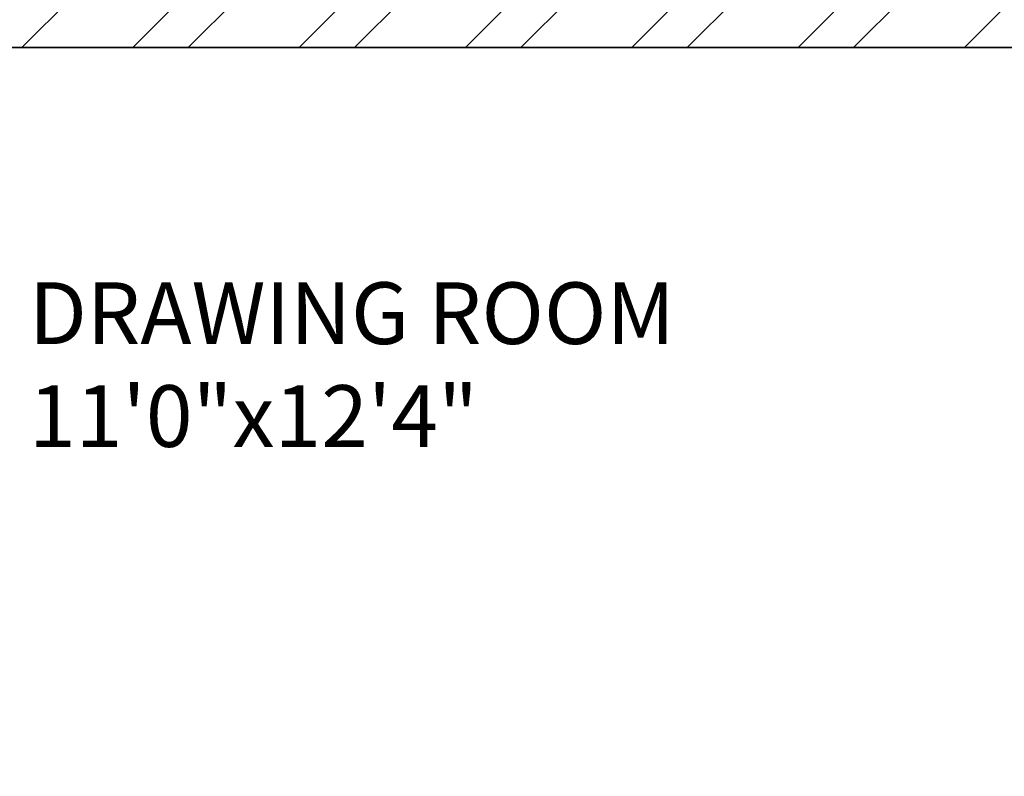
# Model space of a CAD drawing. Units: inches. Extents: x 2168 to 3056, y 1130 to 2629.
# Tile 15 of 42: x 2700 to 2780, y 2017 to 2079. Entities that reach past the tile are written whole.
import ezdxf

# ---------------------------------------------------------------- set-up
doc = ezdxf.new("R2010")
doc.units = ezdxf.units.IN
doc.layers.add('A-AREA-IDEN', color=7, linetype='Continuous', lineweight=18)
doc.layers.add('A-WALL', color=7, linetype='Continuous', lineweight=35)
doc.layers.add('A-WALL-PATT', color=143, linetype='Continuous', lineweight=13, true_color=0x7aafdf)
doc.styles.get("Standard").update_dxf_attribs({"font": 'arial.ttf'})

msp = doc.modelspace()

# ---------------------------------------------------------------- hatches: boundary and pattern name
at = {"layer": 'A-WALL-PATT'}
h = msp.add_hatch(dxfattribs=at)
h.set_pattern_fill('ANSI32', color=256)
h.paths.add_polyline_path([(2463.796, 2409.389), (2467.387, 2409.389), (2467.387, 2413.889), (2454.768, 2413.889), (2454.768, 2411.639), (2454.768, 2409.389), (2459.296, 2409.389), (2459.296, 2265.389), (2455.644, 2265.389), (2455.644, 2260.889), (2467.349, 2260.889), (2467.349, 2263.139), (2467.349, 2265.389), (2463.796, 2265.389)])
h.paths.add_polyline_path([(2431.596, 2413.889), (2409.647, 2413.889), (2409.647, 2409.389), (2431.596, 2409.389), (2431.596, 2411.639)])
h.paths.add_polyline_path([(2349.647, 2413.889), (2331.796, 2413.889), (2331.796, 2362.671), (2336.296, 2362.671), (2336.296, 2409.389), (2349.647, 2409.389), (2349.647, 2411.639)])
h.paths.add_polyline_path([(2634.149, 2411.639), (2634.149, 2413.889), (2562.293, 2413.889), (2562.293, 2409.389), (2595.796, 2409.389), (2595.796, 2280.309), (2595.826, 2280.309), (2595.826, 2265.389), (2499.91, 2265.389), (2499.91, 2260.889), (2550.796, 2260.889), (2550.796, 2117.308), (2555.296, 2117.308), (2555.296, 2168.08), (2571.93, 2168.08), (2571.93, 2176.889), (2559.796, 2176.889), (2559.796, 2256.389), (2640.796, 2256.389), (2640.796, 2176.889), (2626.428, 2176.889), (2626.428, 2168.08), (2645.296, 2168.08), (2645.296, 2116.637), (2649.796, 2116.637), (2649.796, 2260.889), (2691.251, 2260.889), (2691.251, 2263.139), (2691.251, 2265.389), (2670.655, 2265.389), (2670.655, 2265.365), (2600.296, 2265.365), (2600.296, 2280.258), (2600.296, 2409.389), (2634.149, 2409.389)])
h.paths.add_polyline_path([(2600.296, 2473.889), (2612.84, 2473.889), (2612.84, 2478.389), (2572.636, 2478.389), (2572.636, 2473.889), (2595.796, 2473.889), (2595.796, 2413.889), (2600.296, 2413.889)])
h.paths.add_polyline_path([(2535.796, 2473.889), (2548.636, 2473.889), (2548.636, 2478.389), (2531.396, 2478.389), (2531.396, 2413.889), (2521.6, 2413.889), (2521.6, 2409.389), (2539.239, 2409.389), (2539.239, 2411.639), (2539.239, 2413.889), (2535.796, 2413.889)])
h.paths.add_polyline_path([(2664.796, 2478.389), (2636.84, 2478.389), (2636.84, 2473.889), (2660.296, 2473.889), (2660.296, 2413.889), (2656.165, 2413.889), (2656.165, 2409.389), (2671.684, 2409.389), (2671.684, 2411.639), (2671.684, 2413.889), (2664.796, 2413.889)])
h.paths.add_polyline_path([(2705.942, 2413.889), (2695.684, 2413.889), (2695.684, 2409.389), (2705.942, 2409.389)])
h.paths.add_polyline_path([(2741.35, 2413.889), (2728.733, 2413.889), (2728.733, 2411.639), (2728.733, 2409.389), (2732.296, 2409.389), (2732.296, 2265.389), (2725.733, 2265.389), (2725.733, 2260.889), (2740.917, 2260.889), (2740.917, 2263.139), (2740.917, 2265.389), (2736.796, 2265.389), (2736.796, 2409.389), (2741.35, 2409.389)])
h.paths.add_polyline_path([(2785.655, 2413.889), (2764.546, 2413.889), (2764.486, 2409.389), (2785.655, 2409.389), (2785.655, 2411.639)])
h.paths.add_polyline_path([(2864.296, 2413.889), (2845.655, 2413.889), (2845.655, 2409.389), (2859.796, 2409.389), (2859.796, 2368.425), (2864.296, 2368.425)])
h.paths.add_polyline_path([(2864.296, 2308.425), (2862.046, 2308.425), (2859.796, 2308.425), (2859.796, 2265.389), (2774.483, 2265.389), (2774.483, 2263.139), (2774.483, 2260.889), (2781.796, 2260.889), (2781.796, 2226.654), (2786.296, 2226.654), (2786.296, 2260.889), (2859.796, 2260.889), (2859.796, 2241.352), (2864.296, 2241.352)])
h.paths.add_polyline_path([(2864.296, 2217.352), (2862.046, 2217.352), (2859.796, 2217.352), (2859.796, 2200.889), (2786.296, 2200.889), (2786.296, 2205.931), (2784.046, 2205.931), (2781.796, 2205.931), (2781.796, 2150.974), (2786.296, 2150.974), (2786.296, 2161.889), (2859.796, 2161.889), (2859.796, 2144.419), (2864.296, 2144.419)])
h.paths.add_polyline_path([(2859.796, 2196.389), (2859.796, 2166.389), (2786.296, 2166.389), (2786.296, 2196.389)], flags=16)
h.paths.add_polyline_path([(2864.296, 2108.419), (2862.046, 2108.419), (2859.796, 2108.419), (2859.796, 2080.889), (2786.296, 2080.889), (2786.296, 2111.993), (2781.796, 2111.993), (2781.796, 2080.889), (2649.796, 2080.889), (2649.796, 2086.036), (2647.546, 2086.036), (2645.296, 2086.036), (2645.296, 2071.739), (2649.796, 2071.739), (2649.796, 2076.389), (2781.796, 2076.389), (2781.796, 2041.792), (2786.296, 2041.792), (2786.296, 2076.389), (2859.796, 2076.389), (2859.796, 2058.577), (2864.296, 2058.577)])
h.paths.add_polyline_path([(2864.296, 2022.577), (2859.796, 2022.577), (2859.796, 1992.389), (2786.296, 1992.389), (2786.296, 1999.573), (2781.796, 1999.573), (2781.796, 1848.085), (2784.046, 1848.085), (2786.296, 1848.085), (2786.296, 1851.389), (2859.796, 1851.389), (2859.796, 1838.258), (2864.296, 1838.258)], flags=17)
h.paths.add_polyline_path([(2859.796, 1987.889), (2859.796, 1855.889), (2786.296, 1855.889), (2786.296, 1987.889)], flags=16)
h.paths.add_polyline_path([(2823.046, 1987.889), (2841.421, 1921.889), (2823.046, 1855.889)], flags=0)
h.paths.add_polyline_path([(2864.296, 1814.258), (2859.796, 1814.258), (2859.796, 1791.389), (2786.296, 1791.389), (2786.296, 1825.658), (2784.046, 1825.658), (2781.796, 1825.658), (2781.796, 1791.389), (2720.155, 1791.389), (2720.155, 1791.265), (2649.796, 1791.265), (2649.796, 1806.159), (2649.796, 2038.983), (2647.546, 2038.983), (2645.296, 2038.983), (2645.296, 1783.925), (2649.796, 1783.925), (2649.796, 1786.889), (2781.796, 1786.889), (2781.796, 1746.789), (2786.296, 1746.789), (2786.296, 1786.889), (2859.796, 1786.889), (2859.796, 1770.083), (2864.296, 1770.083)])
h.paths.add_polyline_path([(2864.296, 1734.083), (2862.046, 1734.083), (2859.796, 1734.083), (2859.796, 1705.889), (2786.296, 1705.889), (2786.296, 1714.166), (2781.796, 1714.166), (2781.796, 1660.527), (2786.296, 1660.527), (2786.296, 1666.889), (2859.796, 1666.889), (2859.796, 1648.342), (2864.296, 1648.342)])
h.paths.add_polyline_path([(2786.296, 1701.389), (2859.796, 1701.389), (2859.796, 1671.389), (2786.296, 1671.389)], flags=16)
h.paths.add_polyline_path([(2649.796, 1756.576), (2647.546, 1756.576), (2645.296, 1756.576), (2645.296, 1606.889), (2555.296, 1606.889), (2555.296, 1749.513), (2553.046, 1749.513), (2550.796, 1749.513), (2550.796, 1606.889), (2503.006, 1606.889), (2503.006, 1604.639), (2503.006, 1602.389), (2595.796, 1602.389), (2595.849, 1602.389), (2595.849, 1587.495), (2595.796, 1458.389), (2561.502, 1458.389), (2561.502, 1456.139), (2561.502, 1453.889), (2595.796, 1453.889), (2595.796, 1381.889), (2573.438, 1381.889), (2573.438, 1377.389), (2613.01, 1377.389), (2613.01, 1379.639), (2613.01, 1381.889), (2600.296, 1381.889), (2600.296, 1453.889), (2634.327, 1453.889), (2634.327, 1458.389), (2600.296, 1458.389), (2600.296, 1602.389), (2670.655, 1602.389), (2694.095, 1602.389), (2694.095, 1606.889), (2649.796, 1606.889)])
h.paths.add_polyline_path([(2736.796, 1602.389), (2741.562, 1602.389), (2741.562, 1606.889), (2726.203, 1606.889), (2726.203, 1604.639), (2726.203, 1602.389), (2732.296, 1602.389), (2732.296, 1458.389), (2727.899, 1458.389), (2727.899, 1453.889), (2740.821, 1453.889), (2740.821, 1456.139), (2740.821, 1458.389), (2736.796, 1458.389)])
h.paths.add_polyline_path([(2859.796, 1606.889), (2786.296, 1606.889), (2786.296, 1637.334), (2784.046, 1637.334), (2781.796, 1637.334), (2781.796, 1606.889), (2775.612, 1606.889), (2775.612, 1602.389), (2859.796, 1602.389)])
h.paths.add_polyline_path([(2864.296, 1624.342), (2862.046, 1624.342), (2859.796, 1624.342), (2859.796, 1570.39), (2864.296, 1570.39)])
h.paths.add_polyline_path([(2864.296, 1510.39), (2862.046, 1510.39), (2859.796, 1510.39), (2859.796, 1458.389), (2846.735, 1458.389), (2846.735, 1456.139), (2846.735, 1453.889), (2864.296, 1453.889)])
h.paths.add_polyline_path([(2786.735, 1458.389), (2765.444, 1458.389), (2765.444, 1453.889), (2786.735, 1453.889)])
h.paths.add_polyline_path([(2706.004, 1458.389), (2695.36, 1458.389), (2695.36, 1453.889), (2706.004, 1453.889), (2706.004, 1456.139)])
h.paths.add_polyline_path([(2671.36, 1456.139), (2671.36, 1458.389), (2655.986, 1458.389), (2655.986, 1456.139), (2655.986, 1453.889), (2660.296, 1453.889), (2660.296, 1381.889), (2637.01, 1381.889), (2637.01, 1377.389), (2664.796, 1377.389), (2664.796, 1453.889), (2671.36, 1453.889)], flags=17)
h.paths.add_polyline_path([(2539.829, 1458.389), (2520.237, 1458.389), (2520.237, 1453.889), (2531.296, 1453.889), (2531.296, 1377.389), (2546.449, 1377.389), (2546.449, 1379.639), (2546.449, 1381.889), (2535.796, 1381.889), (2535.796, 1453.889), (2539.829, 1453.889)], flags=17)
h.paths.add_polyline_path([(2496.237, 1458.389), (2489.13, 1458.389), (2489.13, 1453.889), (2496.237, 1453.889), (2496.237, 1456.139)])
h.paths.add_polyline_path([(2467.433, 1456.139), (2467.433, 1458.389), (2463.796, 1458.389), (2463.796, 1602.389), (2468.242, 1602.389), (2468.242, 1605.7), (2468.242, 1606.889), (2454.602, 1606.889), (2454.602, 1602.389), (2459.296, 1602.389), (2459.296, 1458.389), (2454.24, 1458.389), (2454.24, 1453.889), (2467.433, 1453.889)])
h.paths.add_polyline_path([(2431.601, 1456.139), (2431.601, 1458.389), (2411.386, 1458.389), (2411.386, 1453.889), (2431.601, 1453.889)])
h.paths.add_polyline_path([(2351.386, 1458.389), (2336.296, 1458.389), (2336.296, 1490.693), (2334.046, 1490.693), (2331.796, 1490.693), (2331.796, 1453.889), (2351.386, 1453.889), (2351.386, 1456.139)])
h.paths.add_polyline_path([(2336.296, 1629.705), (2331.796, 1629.705), (2331.796, 1552.317), (2336.296, 1552.317), (2336.296, 1602.389), (2406.655, 1602.389), (2423.472, 1602.389), (2423.472, 1606.889), (2418.796, 1606.889), (2418.796, 1643.678), (2416.546, 1643.678), (2414.296, 1643.678), (2414.296, 1606.889), (2336.296, 1606.889)])
h.paths.add_polyline_path([(2418.796, 1714.384), (2414.296, 1714.384), (2414.296, 1705.889), (2336.296, 1705.889), (2336.296, 1731.324), (2334.046, 1731.324), (2331.796, 1731.324), (2331.796, 1653.705), (2334.046, 1653.705), (2336.296, 1653.705), (2336.296, 1666.889), (2414.296, 1666.889), (2414.296, 1663.589), (2418.796, 1663.589)])
h.paths.add_polyline_path([(2336.296, 1701.389), (2414.296, 1701.389), (2414.296, 1671.389), (2336.296, 1671.389)], flags=16)
h.paths.add_polyline_path([(2555.296, 2040.059), (2550.796, 2040.059), (2550.796, 1791.389), (2550.561, 1791.205), (2480.202, 1791.205), (2418.796, 1791.389), (2418.796, 1825.448), (2416.546, 1825.448), (2414.296, 1825.448), (2414.296, 1791.389), (2336.296, 1791.389), (2336.296, 1806.409), (2331.796, 1806.409), (2331.796, 1767.324), (2336.296, 1767.324), (2336.296, 1786.889), (2414.296, 1786.889), (2414.296, 1745.457), (2418.796, 1745.457), (2418.796, 1786.889), (2550.796, 1786.889), (2550.796, 1783.011), (2555.296, 1783.011)])
h.paths.add_polyline_path([(2418.796, 1923.389), (2423.207, 1923.389), (2423.207, 1925.639), (2423.207, 1927.889), (2418.796, 1927.889), (2418.796, 2000.048), (2414.296, 2000.048), (2414.296, 1992.389), (2336.296, 1992.389), (2336.296, 1987.889), (2414.296, 1987.889), (2414.296, 1855.889), (2336.296, 1855.889), (2336.296, 1851.389), (2414.296, 1851.389), (2414.296, 1846.759), (2418.796, 1846.759)], flags=17)
h.paths.add_polyline_path([(2336.296, 2019.294), (2334.046, 2019.294), (2331.796, 2019.294), (2331.796, 1830.409), (2336.296, 1830.409)], flags=17)
h.paths.add_polyline_path([(2550.796, 1927.889), (2453.541, 1927.889), (2453.541, 1925.639), (2453.541, 1923.389), (2550.796, 1923.389)], flags=17)
h.paths.add_polyline_path([(2744.987, 1927.889), (2649.796, 1927.889), (2649.796, 1923.389), (2744.987, 1923.389), (2744.987, 1925.639)], flags=17)
h.paths.add_polyline_path([(2555.296, 2086.458), (2553.046, 2086.458), (2550.796, 2086.458), (2550.796, 2080.889), (2418.796, 2080.889), (2336.296, 2080.889), (2336.296, 2115.399), (2334.046, 2115.399), (2331.796, 2115.399), (2331.796, 2055.294), (2336.296, 2055.294), (2336.296, 2076.389), (2550.796, 2076.389), (2550.796, 2071.538), (2555.296, 2071.538)])
h.paths.add_polyline_path([(2418.796, 2121.389), (2414.296, 2121.389), (2414.296, 2080.889), (2418.796, 2080.889)])
h.paths.add_polyline_path([(2418.796, 2076.389), (2414.296, 2076.389), (2414.296, 2035.123), (2418.796, 2035.123)])
h.paths.add_polyline_path([(2422.868, 2263.139), (2422.868, 2265.389), (2406.655, 2265.389), (2406.655, 2265.359), (2336.296, 2265.359), (2336.296, 2280.252), (2336.296, 2302.671), (2334.046, 2302.671), (2331.796, 2302.671), (2331.796, 2246.853), (2336.296, 2246.853), (2336.296, 2260.889), (2414.296, 2260.889), (2414.296, 2223.996), (2418.796, 2223.996), (2418.796, 2260.889), (2422.868, 2260.889)])
h.paths.add_polyline_path([(2418.796, 2204.783), (2416.546, 2204.783), (2414.296, 2204.783), (2414.296, 2200.889), (2336.296, 2200.889), (2336.296, 2220.853), (2331.796, 2220.853), (2331.796, 2151.399), (2336.296, 2151.399), (2336.296, 2161.889), (2414.296, 2161.889), (2414.296, 2153.726), (2418.796, 2153.726)])
h.paths.add_polyline_path([(2414.296, 2196.389), (2414.296, 2166.389), (2336.296, 2166.389), (2336.296, 2196.389)], flags=16)
h.paths.add_polyline_path([(2375.296, 2181.389), (2336.296, 2166.389), (2336.296, 2196.389)], flags=0)
h.paths.add_polyline_path([(2809.595, 2172.34), (2838.804, 2172.34), (2838.804, 2190.997), (2809.595, 2190.997)], flags=8)
h.paths.add_polyline_path([(2849.75, 1919.585), (2849.75, 1952.672), (2831.093, 1952.672), (2831.093, 1919.585)], flags=8)
h.paths.add_polyline_path([(2808.875, 1901.967), (2808.875, 1937.85), (2790.149, 1937.85), (2790.149, 1901.967)], flags=8)
h.paths.add_polyline_path([(2806.285, 1671.896), (2835.493, 1671.896), (2835.493, 1690.553), (2806.285, 1690.553)], flags=8)
h.paths.add_polyline_path([(2353.186, 1676.549), (2382.395, 1676.549), (2382.395, 1695.207), (2353.186, 1695.207)], flags=8)
h.paths.add_polyline_path([(2360.083, 1832.308), (2389.241, 1832.308), (2389.241, 1850.966), (2360.083, 1850.966)], flags=25)
h.paths.add_polyline_path([(2354.822, 2167.823), (2384.031, 2167.823), (2384.031, 2186.481), (2354.822, 2186.481)], flags=8)

# ---------------------------------------------------------------- linework, layer by layer
at = {"layer": 'A-WALL'}
msp.add_line((2649.796, 2076.389), (2781.796, 2076.389), dxfattribs=at)

# ---------------------------------------------------------------- texts
at = {"layer": 'A-AREA-IDEN', "insert": (2701.082, 2057.359), "char_height": 5, "attachment_point": 1}
msp.add_mtext_dynamic_manual_height_columns('DRAWING ROOM\\P11\'0"x12\'4"', width=126.20315, gutter_width=12.5, heights=[0], dxfattribs=at)

doc.saveas('drawing.dxf')
